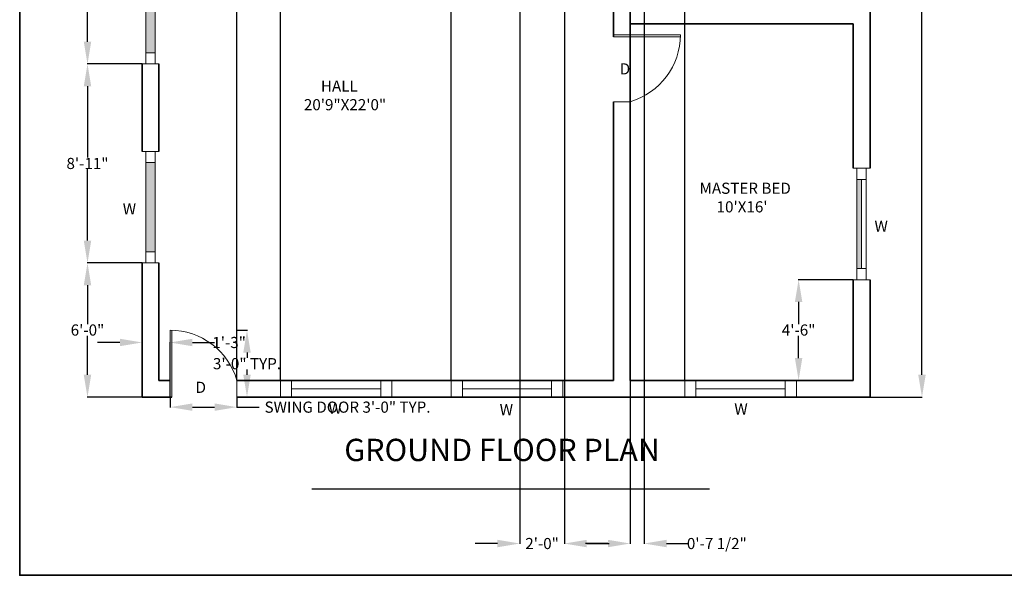
# Model space of a CAD drawing. Units: inches. Extents: x 115 to 1174, y 222 to 1302.
# Tile 1 of 5: x 115 to 644, y 222 to 521. Entities that reach past the tile are written whole.
import ezdxf

# ---------------------------------------------------------------- set-up
doc = ezdxf.new("R2010")
doc.units = ezdxf.units.IN
doc.header["$MEASUREMENT"] = 0
for name, color, linetype, lineweight in [('A-ANNO-DIMS', 2, 'Continuous', 18), ('A-ANNO-IDEN', 7, 'Continuous', 13), ('A-ANNO-TEXT', 7, 'Continuous', 25), ('A-ANNO-TTLB', 7, 'Continuous', 35), ('A-AREA-IDEN', 7, 'Continuous', 18), ('A-DOOR', 3, 'Continuous', 18), ('A-GLAZ', 4, 'Continuous', 18), ('A-GLAZ-PATT', 8, 'Continuous', 13), ('A-WALL', 7, 'Continuous', 35)]:
    doc.layers.add(name, color=color, linetype=linetype, lineweight=lineweight)
doc.styles.get("Standard").update_dxf_attribs({"font": 'arial.ttf'})
doc.dimstyles.get("Standard").update_dxf_attribs({"dimtxt": 6, "dimasz": 12, "dimexe": 0.18, "dimexo": 0.0625, "dimgap": 0.09, "dimtad": 0, "dimtih": 1, "dimtoh": 1, "dimdec": 1, "dimzin": 0, "dimdsep": 46, "dimlunit": 3, "dimtxsty": 'Standard', "dimcen": 0.09, "dimadec": 0, "dimazin": 0, "dimtfac": 1, "dimtdec": 1, "dimtofl": 0, "dimtmove": 0, "dimatfit": 3, "dimfxl": 1, "dimtolj": 1, "dimtzin": 0, "dimarcsym": 0})

# ---------------------------------------------------------------- blocks, each defined once
blk = doc.blocks.new('*D2')
at = {"layer": 'A-ANNO-DIMS', "color": 0, "lineweight": -2, "transparency": 16777216}
for p, q in [((572.28, 801.06), (600.35, 801.06)), ((600.17, 789.06), (600.17, 562.72)), ((600.17, 330.06), (600.17, 556.41)), ((572.28, 318.06), (600.35, 318.06))]:
    blk.add_line(p, q, dxfattribs=at)
at = {"layer": 'A-ANNO-DIMS', "color": 0, "transparency": 16777216}
for points in [[(598.17, 789.06), (602.17, 789.06), (600.17, 801.06)], [(598.17, 330.06), (602.17, 330.06), (600.17, 318.06)]]:
    blk.add_solid(points, dxfattribs=at)
at = {"layer": 'Defpoints', "color": 0, "transparency": 16777216}
for p in [(572.22, 801.06), (572.22, 318.06), (600.17, 318.06)]:
    blk.add_point(p, dxfattribs=at)
at = {"layer": 'A-ANNO-DIMS', "color": 0, "transparency": 16777216, "insert": (600.17, 559.56), "char_height": 6, "attachment_point": 5}
blk.add_mtext('\\A1;40\'-3.0"', dxfattribs=at)
blk = doc.blocks.new('DOOR-36-SWING')
for p, q in [((0, 0), (0, 36)), ((0, 36), (0, 0)), ((1, 36), (1, 0)), ((36, 0), (36, 9)), ((0, 0), (1, 0))]:
    blk.add_line(p, q)
blk.add_arc((0, -1.5), 37.5, 16.2602, 90)
blk = doc.blocks.new('WIN-60-FULL-FRAME')
for p, q in [((0, 0), (0, 9)), ((0, 9), (60, 9)), ((6, 0), (6, 9)), ((54, 9), (54, 0)), ((60, 9), (60, 0)), ((60, 0), (0, 0)), ((54, 4.5), (6, 4.5))]:
    blk.add_line(p, q)
blk = doc.blocks.new('*D17')
at = {"layer": 'A-ANNO-DIMS', "color": 0, "lineweight": -2, "transparency": 16777216}
for p, q in [((195.72, 318), (195.72, 312.48)), ((231.72, 318), (231.72, 312.48)), ((207.72, 312.66), (219.72, 312.66)), ((231.72, 312.66), (243.72, 312.66))]:
    blk.add_line(p, q, dxfattribs=at)
at = {"layer": 'A-ANNO-DIMS', "color": 0, "transparency": 16777216}
for points in [[(207.72, 314.66), (207.72, 310.66), (195.72, 312.66)], [(219.72, 314.66), (219.72, 310.66), (231.72, 312.66)]]:
    blk.add_solid(points, dxfattribs=at)
at = {"layer": 'Defpoints', "color": 0, "transparency": 16777216}
for p in [(195.72, 318.06), (231.72, 318.06), (231.72, 312.66)]:
    blk.add_point(p, dxfattribs=at)
at = {"layer": 'A-ANNO-DIMS', "color": 0, "transparency": 16777216, "insert": (291.19, 312.66), "char_height": 6, "attachment_point": 5}
blk.add_mtext('\\A1;SWING DOOR 3\'-0" TYP.', dxfattribs=at)
blk = doc.blocks.new('*D18')
at = {"layer": 'A-ANNO-DIMS', "color": 0, "lineweight": -2, "transparency": 16777216}
for p, q in [((231.78, 354.06), (237.3, 354.06)), ((237.12, 342.06), (237.12, 339.22)), ((237.12, 330.06), (237.12, 332.91)), ((231.78, 318.06), (237.3, 318.06))]:
    blk.add_line(p, q, dxfattribs=at)
at = {"layer": 'A-ANNO-DIMS', "color": 0, "transparency": 16777216}
for points in [[(235.12, 342.06), (239.12, 342.06), (237.12, 354.06)], [(235.12, 330.06), (239.12, 330.06), (237.12, 318.06)]]:
    blk.add_solid(points, dxfattribs=at)
at = {"layer": 'Defpoints', "color": 0, "transparency": 16777216}
for p in [(231.72, 354.06), (237.12, 354.06), (231.72, 318.06)]:
    blk.add_point(p, dxfattribs=at)
at = {"layer": 'A-ANNO-DIMS', "color": 0, "transparency": 16777216, "insert": (237.12, 336.06), "char_height": 6, "attachment_point": 5}
blk.add_mtext('\\A1;3\'-0" TYP.', dxfattribs=at)
blk = doc.blocks.new('*D37')
at = {"layer": 'A-ANNO-DIMS', "color": 0, "lineweight": -2, "transparency": 16777216}
for p, q in [((180.66, 390.28), (151.14, 390.28)), ((151.32, 378.28), (151.32, 357.32)), ((151.32, 330.06), (151.32, 351.02)), ((180.66, 318.06), (151.14, 318.06))]:
    blk.add_line(p, q, dxfattribs=at)
at = {"layer": 'A-ANNO-DIMS', "color": 0, "transparency": 16777216}
for points in [[(149.32, 378.28), (153.32, 378.28), (151.32, 390.28)], [(149.32, 330.06), (153.32, 330.06), (151.32, 318.06)]]:
    blk.add_solid(points, dxfattribs=at)
at = {"layer": 'Defpoints', "color": 0, "transparency": 16777216}
for p in [(151.32, 390.28), (180.72, 390.28), (180.72, 318.06)]:
    blk.add_point(p, dxfattribs=at)
at = {"layer": 'A-ANNO-DIMS', "color": 0, "transparency": 16777216, "insert": (151.32, 354.17), "char_height": 6, "attachment_point": 5}
blk.add_mtext('\\A1;6\'-0"', dxfattribs=at)
blk = doc.blocks.new('*D38')
at = {"layer": 'A-ANNO-DIMS', "color": 0, "lineweight": -2, "transparency": 16777216}
for p, q in [((180.66, 497.36), (151.14, 497.36)), ((151.32, 485.36), (151.32, 446.97)), ((151.32, 402.28), (151.32, 440.67)), ((180.66, 390.28), (151.14, 390.28))]:
    blk.add_line(p, q, dxfattribs=at)
at = {"layer": 'A-ANNO-DIMS', "color": 0, "transparency": 16777216}
for points in [[(149.32, 485.36), (153.32, 485.36), (151.32, 497.36)], [(149.32, 402.28), (153.32, 402.28), (151.32, 390.28)]]:
    blk.add_solid(points, dxfattribs=at)
at = {"layer": 'Defpoints', "color": 0, "transparency": 16777216}
for p in [(151.32, 497.36), (180.72, 497.36), (180.72, 390.28)]:
    blk.add_point(p, dxfattribs=at)
at = {"layer": 'A-ANNO-DIMS', "color": 0, "transparency": 16777216, "insert": (151.32, 443.82), "char_height": 6, "attachment_point": 5}
blk.add_mtext('\\A1;8\'-11"', dxfattribs=at)
blk = doc.blocks.new('*D39')
at = {"layer": 'A-ANNO-DIMS', "color": 0, "lineweight": -2, "transparency": 16777216}
for p, q in [((180.66, 641.84), (151.14, 641.84)), ((151.32, 629.84), (151.32, 572.79)), ((151.32, 509.36), (151.32, 566.41)), ((180.66, 497.36), (151.14, 497.36))]:
    blk.add_line(p, q, dxfattribs=at)
at = {"layer": 'A-ANNO-DIMS', "color": 0, "transparency": 16777216}
for points in [[(149.32, 629.84), (153.32, 629.84), (151.32, 641.84)], [(149.32, 509.36), (153.32, 509.36), (151.32, 497.36)]]:
    blk.add_solid(points, dxfattribs=at)
at = {"layer": 'Defpoints', "color": 0, "transparency": 16777216}
for p in [(151.32, 641.84), (180.72, 641.84), (180.72, 497.36)]:
    blk.add_point(p, dxfattribs=at)
at = {"layer": 'A-ANNO-DIMS', "color": 0, "transparency": 16777216, "insert": (151.32, 569.6), "char_height": 6, "attachment_point": 5}
blk.add_mtext('\\A1;12\'-0 1/2"', dxfattribs=at)
blk = doc.blocks.new('*D41')
at = {"layer": 'A-ANNO-DIMS', "color": 0, "lineweight": -2, "transparency": 16777216}
for p, q in [((563.16, 381.27), (533.64, 381.27)), ((533.82, 369.27), (533.82, 357.32)), ((533.82, 339.06), (533.82, 351.02)), ((563.16, 327.06), (533.64, 327.06))]:
    blk.add_line(p, q, dxfattribs=at)
at = {"layer": 'A-ANNO-DIMS', "color": 0, "transparency": 16777216}
for points in [[(531.82, 369.27), (535.82, 369.27), (533.82, 381.27)], [(531.82, 339.06), (535.82, 339.06), (533.82, 327.06)]]:
    blk.add_solid(points, dxfattribs=at)
at = {"layer": 'Defpoints', "color": 0, "transparency": 16777216}
for p in [(533.82, 381.27), (563.22, 381.27), (563.22, 327.06)]:
    blk.add_point(p, dxfattribs=at)
at = {"layer": 'A-ANNO-DIMS', "color": 0, "transparency": 16777216, "insert": (533.82, 354.17), "char_height": 6, "attachment_point": 5}
blk.add_mtext('\\A1;4\'-6"', dxfattribs=at)
blk = doc.blocks.new('*D45')
at = {"layer": 'A-ANNO-DIMS', "color": 0, "lineweight": -2, "transparency": 16777216}
for p, q in [((383.829365, 792.001973), (383.829365, 239.058512)), ((407.829365, 792.001973), (407.829365, 239.058512)), ((371.829365, 239.238512), (359.829365, 239.238512)), ((419.829365, 239.238512), (431.829365, 239.238512))]:
    blk.add_line(p, q, dxfattribs=at)
at = {"layer": 'A-ANNO-DIMS', "color": 0, "transparency": 16777216}
for points in [[(371.829365, 241.238512), (371.829365, 237.238512), (383.829365, 239.238512)], [(419.829365, 241.238512), (419.829365, 237.238512), (407.829365, 239.238512)]]:
    blk.add_solid(points, dxfattribs=at)
at = {"layer": 'Defpoints', "color": 0, "transparency": 16777216}
for p in [(383.829365, 792.064473), (407.829365, 792.064473), (407.829365, 239.238512)]:
    blk.add_point(p, dxfattribs=at)
at = {"layer": 'A-ANNO-DIMS', "color": 0, "transparency": 16777216, "insert": (395.829365, 239.238512), "char_height": 6, "attachment_point": 5}
blk.add_mtext('\\A1;2\'-0"', dxfattribs=at)
blk = doc.blocks.new('*D46')
at = {"layer": 'A-ANNO-DIMS', "color": 0, "lineweight": -2, "transparency": 16777216}
for p, q in [((443.22, 792), (443.22, 239.06)), ((450.77, 792), (450.77, 239.06)), ((431.22, 239.24), (419.22, 239.24)), ((462.77, 239.24), (474.77, 239.24))]:
    blk.add_line(p, q, dxfattribs=at)
at = {"layer": 'A-ANNO-DIMS', "color": 0, "transparency": 16777216}
for points in [[(431.22, 241.24), (431.22, 237.24), (443.22, 239.24)], [(462.77, 241.24), (462.77, 237.24), (450.77, 239.24)]]:
    blk.add_solid(points, dxfattribs=at)
at = {"layer": 'Defpoints', "color": 0, "transparency": 16777216}
for p in [(443.22, 792.06), (450.77, 792.06), (450.77, 239.24)]:
    blk.add_point(p, dxfattribs=at)
at = {"layer": 'A-ANNO-DIMS', "color": 0, "transparency": 16777216, "insert": (489.83, 239.24), "char_height": 6, "attachment_point": 5}
blk.add_mtext('\\A1;0\'-7 1/2"', dxfattribs=at)
blk = doc.blocks.new('*D47')
at = {"layer": 'A-ANNO-DIMS', "color": 0, "lineweight": -2, "transparency": 16777216}
for p, q in [((168.72, 347.46), (156.72, 347.46)), ((180.72, 318.13), (180.72, 347.64)), ((195.72, 318.13), (195.72, 347.64)), ((207.72, 347.46), (219.72, 347.46))]:
    blk.add_line(p, q, dxfattribs=at)
at = {"layer": 'A-ANNO-DIMS', "color": 0, "transparency": 16777216}
for points in [[(168.72, 349.46), (168.72, 345.46), (180.72, 347.46)], [(207.72, 349.46), (207.72, 345.46), (195.72, 347.46)]]:
    blk.add_solid(points, dxfattribs=at)
at = {"layer": 'Defpoints', "color": 0, "transparency": 16777216}
for p in [(195.72, 347.46), (180.72, 318.06), (195.72, 318.06)]:
    blk.add_point(p, dxfattribs=at)
at = {"layer": 'A-ANNO-DIMS', "color": 0, "transparency": 16777216, "insert": (227.5, 347.46), "char_height": 6, "attachment_point": 5}
blk.add_mtext('\\A1;1\'-3"', dxfattribs=at)
blk = doc.blocks.new('*D48')
at = {"layer": 'A-ANNO-DIMS', "color": 0, "lineweight": -2, "transparency": 16777216}
for p, q in [((219.72, 830.46), (207.72, 830.46)), ((231.72, 327.13), (231.72, 830.64)), ((255.09, 327.13), (255.09, 830.64)), ((267.09, 830.46), (279.09, 830.46))]:
    blk.add_line(p, q, dxfattribs=at)
at = {"layer": 'A-ANNO-DIMS', "color": 0, "transparency": 16777216}
for points in [[(219.72, 832.46), (219.72, 828.46), (231.72, 830.46)], [(267.09, 832.46), (267.09, 828.46), (255.09, 830.46)]]:
    blk.add_solid(points, dxfattribs=at)
at = {"layer": 'Defpoints', "color": 0, "transparency": 16777216}
for p in [(255.09, 830.46), (231.72, 327.06), (255.09, 327.06)]:
    blk.add_point(p, dxfattribs=at)
at = {"layer": 'A-ANNO-DIMS', "color": 0, "transparency": 16777216, "insert": (296.19, 830.46), "char_height": 6, "attachment_point": 5}
blk.add_mtext('\\A1;1\'-11 1/2"', dxfattribs=at)
blk = doc.blocks.new('*D49')
at = {"layer": 'A-ANNO-DIMS', "color": 0, "lineweight": -2, "transparency": 16777216}
for p, q in [((255.09, 327.13), (255.09, 830.64)), ((267.09, 830.46), (292.98, 830.46)), ((334.96, 830.46), (309.06, 830.46)), ((346.96, 327.13), (346.96, 830.64))]:
    blk.add_line(p, q, dxfattribs=at)
at = {"layer": 'A-ANNO-DIMS', "color": 0, "transparency": 16777216}
for points in [[(267.09, 832.46), (267.09, 828.46), (255.09, 830.46)], [(334.96, 832.46), (334.96, 828.46), (346.96, 830.46)]]:
    blk.add_solid(points, dxfattribs=at)
at = {"layer": 'Defpoints', "color": 0, "transparency": 16777216}
for p in [(346.96, 830.46), (255.09, 327.06), (346.96, 327.06)]:
    blk.add_point(p, dxfattribs=at)
at = {"layer": 'A-ANNO-DIMS', "color": 0, "transparency": 16777216, "insert": (301.02, 830.46), "char_height": 6, "attachment_point": 5}
blk.add_mtext('\\A1;7\'-8"', dxfattribs=at)
blk = doc.blocks.new('*D50')
at = {"layer": 'A-ANNO-DIMS', "color": 0, "lineweight": -2, "transparency": 16777216}
for p, q in [((443.22, 327.13), (443.22, 830.64)), ((455.22, 830.46), (460.61, 830.46)), ((472.61, 327.13), (472.61, 830.64)), ((472.61, 830.46), (484.61, 830.46))]:
    blk.add_line(p, q, dxfattribs=at)
at = {"layer": 'A-ANNO-DIMS', "color": 0, "transparency": 16777216}
for points in [[(455.22, 832.46), (455.22, 828.46), (443.22, 830.46)], [(460.61, 832.46), (460.61, 828.46), (472.61, 830.46)]]:
    blk.add_solid(points, dxfattribs=at)
at = {"layer": 'Defpoints', "color": 0, "transparency": 16777216}
for p in [(472.61, 830.46), (443.22, 327.06), (472.61, 327.06)]:
    blk.add_point(p, dxfattribs=at)
at = {"layer": 'A-ANNO-DIMS', "color": 0, "transparency": 16777216, "insert": (499.71, 830.46), "char_height": 6, "attachment_point": 5}
blk.add_mtext('\\A1;2\'-5 1/2"', dxfattribs=at)

msp = doc.modelspace()

# ---------------------------------------------------------------- hatches: boundary and pattern name
at = {"layer": 'A-GLAZ-PATT'}
h = msp.add_hatch(color=256, dxfattribs=at)
h.dxf.hatch_style = 1
h.paths.add_polyline_path([(407.83, 799.06), (383.83, 799.06), (383.83, 794.06), (407.83, 794.06)])
h.paths.add_polyline_path([(567.72, 662.55), (565.22, 662.55), (565.22, 614.55), (567.72, 614.55)])
h.paths.add_polyline_path([(567.72, 435.27), (565.22, 435.27), (565.22, 387.27), (567.72, 387.27)])
h.paths.add_polyline_path([(187.72, 444.28), (182.72, 444.28), (182.72, 396.28), (187.72, 396.28)])
h.paths.add_polyline_path([(187.72, 551.36), (182.72, 551.36), (182.72, 503.36), (187.72, 503.36)])
h.paths.add_polyline_path([(187.72, 695.84), (182.72, 695.84), (182.72, 647.84), (187.72, 647.84)])

# ---------------------------------------------------------------- linework, layer by layer
at = {"layer": 'A-ANNO-TEXT'}
msp.add_line((272.02, 268.64), (485.81, 268.64), dxfattribs=at)
at = {"layer": 'A-ANNO-TTLB'}
msp.add_lwpolyline([(114.85, 1302.15), (1174.06, 1302.15), (1174.06, 222.13), (114.85, 222.13)], close=True, dxfattribs=at)
at = {"layer": 'A-GLAZ'}
for p, q in [((182.72, 497.36), (182.72, 557.36)), ((187.72, 557.36), (187.72, 497.36)), ((187.72, 503.36), (182.72, 503.36)), ((189.72, 497.36), (180.72, 497.36)), ((180.72, 450.28), (189.72, 450.28)), ((182.72, 390.28), (182.72, 450.28)), ((187.72, 450.28), (187.72, 390.28)), ((182.72, 444.28), (187.72, 444.28)), ((563.22, 441.27), (572.22, 441.27)), ((565.22, 381.27), (565.22, 441.27)), ((570.22, 441.27), (570.22, 381.27)), ((565.22, 435.27), (570.22, 435.27)), ((567.72, 435.27), (567.72, 387.27)), ((187.72, 396.28), (182.72, 396.28)), ((189.72, 390.28), (180.72, 390.28)), ((570.22, 387.27), (565.22, 387.27)), ((572.22, 381.27), (563.22, 381.27))]:
    msp.add_line(p, q, dxfattribs=at)
at = {"layer": 'A-WALL'}
for p, q in [((572.22, 608.55), (572.22, 441.27)), ((434.22, 591.06), (434.22, 512.06)), ((434.22, 519.06), (434.22, 513.06)), ((443.22, 519.06), (563.22, 519.06)), ((443.22, 519.06), (443.22, 513.06)), ((563.22, 519.06), (563.22, 441.27)), ((180.72, 497.36), (180.72, 450.28)), ((189.72, 497.36), (189.72, 450.28)), ((434.22, 477.06), (434.22, 327.06)), ((443.22, 477.06), (443.22, 327.06)), ((180.72, 390.28), (180.72, 318.06)), ((189.72, 390.28), (189.72, 327.06)), ((563.22, 381.27), (563.22, 327.06)), ((572.22, 381.27), (572.22, 318.06)), ((189.72, 327.06), (195.72, 327.06)), ((231.72, 327.06), (434.22, 327.06)), ((443.22, 327.06), (563.22, 327.06)), ((180.72, 318.06), (196.72, 318.06)), ((189.72, 318.06), (195.72, 318.06)), ((231.72, 318.06), (572.22, 318.06))]:
    msp.add_line(p, q, dxfattribs=at)

# ---------------------------------------------------------------- block references
at = {"layer": 'A-DOOR', "rotation": 270.0000000000001}
msp.add_blockref('DOOR-36-SWING', (434.22, 513.06), dxfattribs=at)
at = {"layer": 'A-DOOR'}
msp.add_blockref('DOOR-36-SWING', (195.72, 318.06), dxfattribs=at)
at = {"layer": 'A-GLAZ'}
for p in [(255.09, 318.06), (346.96, 318.06), (472.61, 318.06)]:
    msp.add_blockref('WIN-60-FULL-FRAME', p, dxfattribs=at)

# ---------------------------------------------------------------- texts
at = {"layer": 'A-ANNO-IDEN', "char_height": 6, "attachment_point": 1}
for s, width, insert in [('D', 9.3758, (437.59, 497.74)), ('W', 10.5593, (170.28, 422.41)), ('W', 10.5593, (574.62, 413.03)), ('D', 9.3758, (209.44, 326.33)), ('W', 10.5593, (280.92, 315.12)), ('W', 10.5593, (373.02, 314.32)), ('W', 10.5593, (499.23, 314.63))]:
    msp.add_mtext_dynamic_manual_height_columns(s, width=width, gutter_width=30, heights=[0], dxfattribs=dict(at, insert=insert))
at = {"layer": 'A-ANNO-TEXT', "insert": (289.45, 295.63), "char_height": 12, "attachment_point": 1}
msp.add_mtext_dynamic_manual_height_columns('GROUND FLOOR PLAN', width=219.1229, gutter_width=30, heights=[0], dxfattribs=at)
at = {"layer": 'A-AREA-IDEN', "char_height": 6, "attachment_point": 1}
for s, width, insert in [('     HALL\\P20\'9"X22\'0"', 88.4292, (267.71, 488.46)), ("MASTER BED\\P     10'X16'", 126.6157, (480.54, 433.48))]:
    msp.add_mtext_dynamic_manual_height_columns(s, width=width, gutter_width=30, heights=[0], dxfattribs=dict(at, insert=insert))

# ---------------------------------------------------------------- dimensions: what is measured, and where the dimension line sits
at = {"layer": 'A-ANNO-DIMS'}
for base, p1, p2, picture, middle in [((255.09, 830.46), (231.72, 327.06), (255.09, 327.06), '*D48', (296.19, 830.46)), ((472.61, 830.46), (443.22, 327.06), (472.61, 327.06), '*D50', (499.71, 830.46)), ((346.96, 830.46), (255.09, 327.06), (346.96, 327.06), '*D49', (301.02, 830.46)), ((407.83, 239.24), (383.83, 792.06), (407.83, 792.06), '*D45', (395.83, 239.24)), ((450.7739, 239.2385), (443.2197, 792.0645), (450.7739, 792.0645), '*D46', (489.8291, 239.2385)), ((195.72, 347.46), (180.72, 318.06), (195.72, 318.06), '*D47', (227.5, 347.46))]:
    dim = msp.add_linear_dim(base=base, p1=p1, p2=p2, dimstyle='Standard', override={"dimdec": 1, "dimlfac": 1, "dimrnd": 0, "dimzin": 1, "dimdsep": 46, "dimlunit": 4, "dimfrac": 2}, dxfattribs=at)
    dim.commit()
    dim.dimension.update_dxf_attribs({"geometry": picture, "text_midpoint": middle})
for base, p1, p2, override, picture, middle in [((600.17, 318.06), (572.22, 801.06), (572.22, 318.06), {"dimclrd": 0, "dimclre": 0, "dimclrt": 0}, '*D2', (600.17, 559.56)), ((151.32, 641.84), (180.72, 497.36), (180.72, 641.84), {"dimdec": 1, "dimlfac": 1, "dimrnd": 0, "dimzin": 1, "dimdsep": 46, "dimlunit": 4, "dimfrac": 2}, '*D39', (151.32, 569.6)), ((151.32, 497.36), (180.72, 390.28), (180.72, 497.36), {"dimdec": 1, "dimlfac": 1, "dimrnd": 0, "dimzin": 1, "dimdsep": 46, "dimlunit": 4, "dimfrac": 2}, '*D38', (151.32, 443.82)), ((151.32, 390.28), (180.72, 318.06), (180.72, 390.28), {"dimdec": 1, "dimlfac": 1, "dimrnd": 0, "dimzin": 1, "dimdsep": 46, "dimlunit": 4, "dimfrac": 2}, '*D37', (151.32, 354.17)), ((533.82, 381.27), (563.22, 327.06), (563.22, 381.27), {"dimdec": 1, "dimlfac": 1, "dimrnd": 0, "dimzin": 1, "dimdsep": 46, "dimlunit": 4, "dimfrac": 2}, '*D41', (533.82, 354.17))]:
    dim = msp.add_linear_dim(base=base, p1=p1, p2=p2, angle=90, dimstyle='Standard', override=override, dxfattribs=at)
    dim.commit()
    dim.dimension.update_dxf_attribs({"geometry": picture, "text_midpoint": middle})
dim = msp.add_linear_dim(base=(237.12, 354.06), p1=(231.72, 318.06), p2=(231.72, 354.06), angle=90, text='<> TYP.', dimstyle='Standard', override={"dimdec": 1, "dimlfac": 1, "dimrnd": 0, "dimzin": 1, "dimdsep": 46, "dimlunit": 4, "dimfrac": 2}, dxfattribs=at)
dim.commit()
dim.dimension.update_dxf_attribs({"geometry": '*D18', "text_midpoint": (237.12, 336.06)})
dim = msp.add_linear_dim(base=(231.72, 312.66), p1=(195.72, 318.06), p2=(231.72, 318.06), text='SWING DOOR <> TYP.', dimstyle='Standard', override={"dimdec": 1, "dimlfac": 1, "dimrnd": 0, "dimzin": 1, "dimdsep": 46, "dimlunit": 4, "dimfrac": 2}, dxfattribs=at)
dim.commit()
dim.dimension.update_dxf_attribs({"geometry": '*D17', "text_midpoint": (291.19, 312.66)})

doc.saveas('drawing.dxf')
